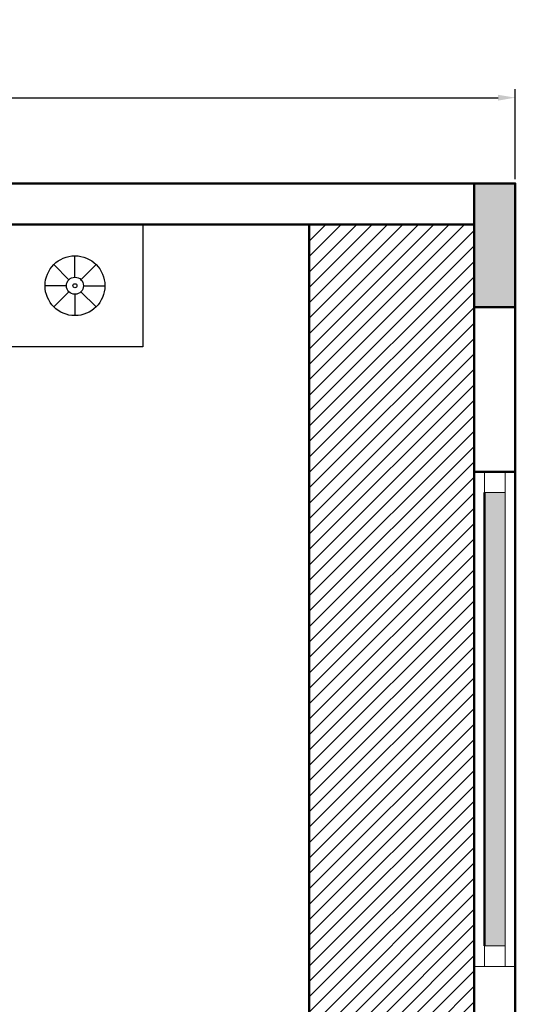
# Model space of a CAD drawing. Units: inches. Extents: x 3064 to 19385, y 846 to 15425.
# Tile 24 of 108: x 3917 to 3989, y 1277 to 1420. Entities that reach past the tile are written whole.
import ezdxf

# ---------------------------------------------------------------- set-up
doc = ezdxf.new("R2010")
doc.units = ezdxf.units.IN
for name, color, linetype, lineweight in [('A-ANNO-DIMS', 2, 'Continuous', 18), ('A-COLS', 1, 'Continuous', 35), ('A-FLOR-FIXT', 9, 'Continuous', 18), ('A-FURN-PATT', 252, 'Continuous', 13), ('A-GLAZ', 4, 'Continuous', 18), ('A-WALL', 7, 'Continuous', 50)]:
    doc.layers.add(name, color=color, linetype=linetype, lineweight=lineweight)
doc.layers.add('BLOCK', color=6, linetype='Continuous')
doc.styles.get("Standard").update_dxf_attribs({"font": 'arial.ttf'})
doc.dimstyles.new('ISO-25', dxfattribs={"dimtxt": 9, "dimasz": 2.5, "dimexe": 1.25, "dimexo": 0.625, "dimtad": 1, "dimdec": 1, "dimlunit": 3, "dimtxsty": 'Standard', "dimcen": 2.5, "dimadec": 0, "dimazin": 0, "dimtfac": 1, "dimtdec": 1, "dimtmove": 0, "dimatfit": 3, "dimfxl": 1, "dimarcsym": 0})

# ---------------------------------------------------------------- blocks, each defined once
blk = doc.blocks.new('A$C52E67D0D')
at = {"layer": 'BLOCK'}
for p, q in [((2251.5, 1605.5), (2251.5, 1684.7)), ((2229.3, 1596.3), (2173.3, 1652.3)), ((2273.7, 1596.3), (2329.7, 1652.3)), ((2220.1, 1574.1), (2140.9, 1574.1)), ((2282.9, 1574.1), (2362.1, 1574.1)), ((2229.3, 1551.9), (2173.3, 1495.9)), ((2251.5, 1542.8), (2251.5, 1463.5)), ((2273.7, 1551.9), (2329.7, 1495.9))]:
    blk.add_line(p, q, dxfattribs=at)
blk.add_lwpolyline([(2001, 1348.6), (2001, 1799.6), (2502, 1799.6), (2502, 1348.6)], close=True, dxfattribs=at)
for radius in [110.6, 31.4, 7.46]:
    blk.add_circle((2251.5, 1574.1), radius, dxfattribs=at)
blk = doc.blocks.new('*D41')
at = {"layer": 'A-ANNO-DIMS', "color": 0, "lineweight": -2, "transparency": 16777216}
for p, q in [((3647.36, 1396.96), (3647.36, 1410.06)), ((3989.36, 1396.96), (3989.36, 1410.06)), ((3649.86, 1408.81), (3986.86, 1408.81))]:
    blk.add_line(p, q, dxfattribs=at)
at = {"layer": 'A-ANNO-DIMS', "color": 0, "transparency": 16777216}
for points in [[(3649.86, 1409.23), (3649.86, 1408.39), (3647.36, 1408.81)], [(3986.86, 1409.23), (3986.86, 1408.39), (3989.36, 1408.81)]]:
    blk.add_solid(points, dxfattribs=at)
at = {"layer": 'Defpoints', "color": 0, "transparency": 16777216}
for p in [(3989.36, 1408.81), (3647.36, 1396.34), (3989.36, 1396.34)]:
    blk.add_point(p, dxfattribs=at)
at = {"layer": 'A-ANNO-DIMS', "color": 0, "transparency": 16777216, "insert": (3818.36, 1414.03), "char_height": 9, "attachment_point": 5}
blk.add_mtext('28\'-6"', dxfattribs=at)
blk = doc.blocks.new('WIN-1900')
blk.add_line((3, 0), (3, 66))
blk.add_lwpolyline([(3, 66), (0, 66), (0, 69), (3, 69)], close=True)

msp = doc.modelspace()

# ---------------------------------------------------------------- hatches: boundary and pattern name
at = {"layer": 'A-COLS'}
h = msp.add_hatch(color=256, dxfattribs=at)
h.dxf.hatch_style = 1
h.paths.add_polyline_path([(3983.36, 1378.34), (3989.36, 1378.34), (3989.36, 1396.34), (3983.36, 1396.34)])
at = {"layer": 'A-FURN-PATT'}
h = msp.add_hatch(dxfattribs=at)
h.set_pattern_fill('ANSI31', color=256, scale=0.5)
h.set_pattern_definition([(45, (-695.1336, 0), (-1.122532, 1.122532), [])])
h.paths.add_polyline_path([(3959.36, 1258.34), (3983.36, 1258.34), (3983.36, 1390.34), (3959.36, 1390.34)])
at = {"layer": 'A-GLAZ'}
h = msp.add_hatch(color=256, dxfattribs=at)
h.dxf.hatch_style = 1
h.paths.add_polyline_path([(3984.86, 1285.34), (3987.86, 1285.34), (3987.86, 1351.34), (3984.86, 1351.34)])

# ---------------------------------------------------------------- linework, layer by layer
msp.add_line((3989.36, 1282.34), (3983.36, 1282.34), dxfattribs=at)
msp.add_lwpolyline([(3987.86, 1282.34), (3984.86, 1282.34), (3984.86, 1285.34), (3987.86, 1285.34)], close=True, dxfattribs=at)
at = {"layer": 'A-WALL'}
for p, q in [((3989.36, 1396.34), (3647.36, 1396.34)), ((3989.36, 904.34), (3989.36, 1396.34)), ((3983.36, 1390.34), (3788.36, 1390.34)), ((3959.36, 1258.34), (3959.36, 1390.34)), ((3983.36, 1258.34), (3983.36, 1390.34)), ((3983.36, 1354.34), (3989.36, 1354.34)), ((3984.86, 1351.34), (3984.86, 1285.34))]:
    msp.add_line(p, q, dxfattribs=at)
msp.add_lwpolyline([(3989.36, 1378.34), (3989.36, 1396.34), (3983.36, 1396.34), (3983.36, 1378.34)], close=True, dxfattribs=at)

# ---------------------------------------------------------------- block references
at = {"layer": 'A-FLOR-FIXT', "xscale": 0.039370099999992, "yscale": 0.039370099999992, "zscale": 0.039370099999992}
msp.add_blockref('A$C52E67D0D', (3836.61, 1319.47), dxfattribs=at)
at = {"layer": 'A-GLAZ'}
msp.add_blockref('WIN-1900', (3984.86, 1285.34), dxfattribs=at)

# ---------------------------------------------------------------- dimensions: what is measured, and where the dimension line sits
at = {"layer": 'A-ANNO-DIMS'}
dim = msp.add_linear_dim(base=(3989.36, 1408.81), p1=(3647.36, 1396.34), p2=(3989.36, 1396.34), dimstyle='ISO-25', override={"dimclrd": 0, "dimclre": 0, "dimclrt": 0}, dxfattribs=at)
dim.commit()
dim.dimension.update_dxf_attribs({"geometry": '*D41', "text_midpoint": (3818.36, 1414.03)})

doc.saveas('drawing.dxf')
